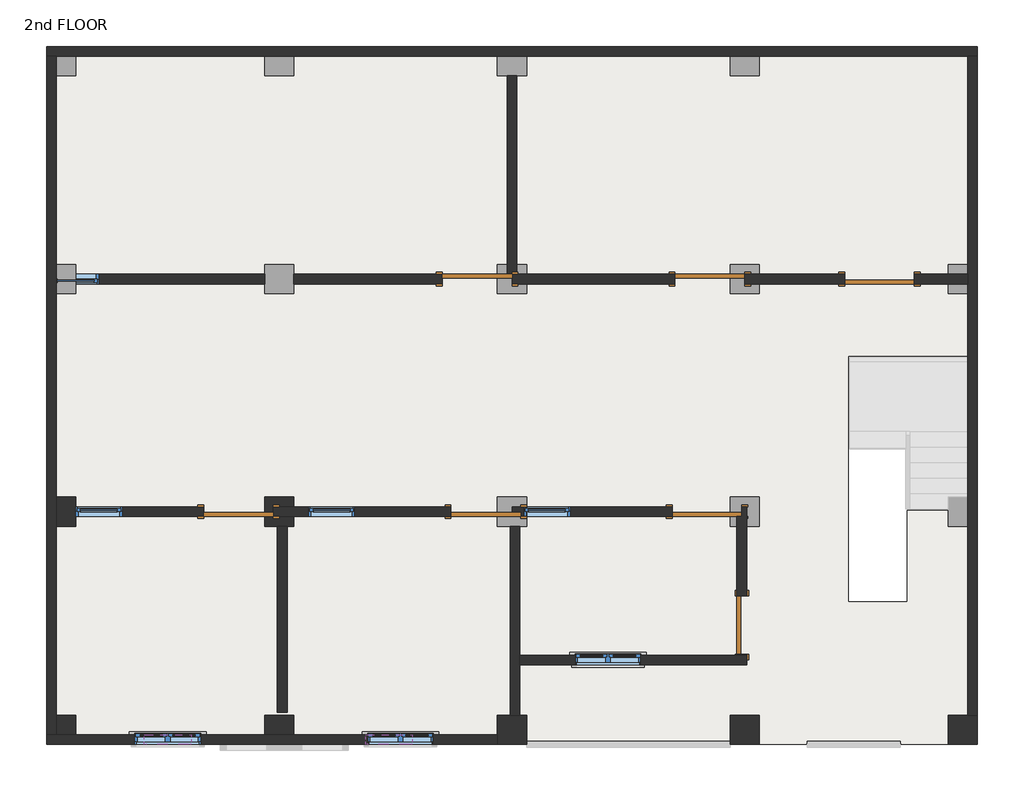
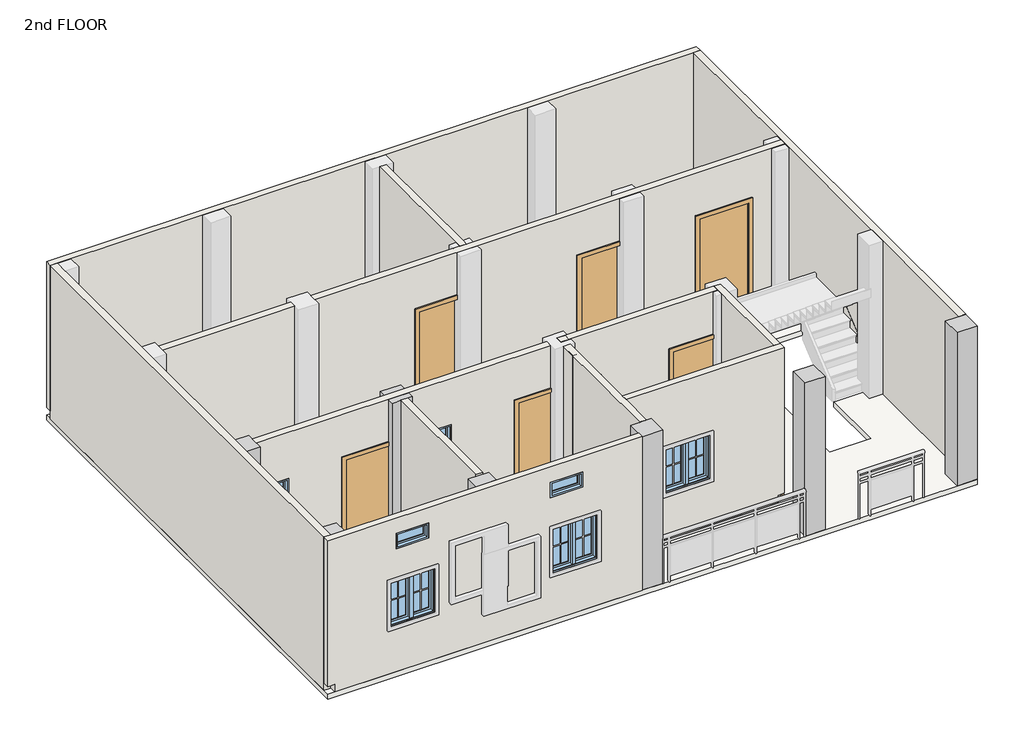
# One storey, part 1 of 2: 15 walls, 9 windows, 7 columns, 7 doors, 1 slab.
"""IFC4 building model written with IfcOpenShell, lengths in millimetres."""

from ifc_helpers import new_model, si_unit, frame, origin, place, context, project, spatial, polyline, outline, extrude, faceted_brep, transform, mapped, element, save
from components import door_e00f436c, door_a1797ceb, window_4c2727af, window_0bf3737e, window_78893e6c, window_0d9958e7

model = new_model("IFC4")

# Units and contexts
model_context = context("Model", 3, world=origin())
ifc_project = project(units=[si_unit("LENGTHUNIT", "METRE", prefix="MILLI")], contexts=[model_context])

# Site, building, storey
site = spatial("IfcSite", under=ifc_project)
building = spatial("IfcBuilding", under=site)
storey = spatial("IfcBuildingStorey", under=building, Name="2nd FLOOR", Elevation=5943.6)

# Columns
placement = place(None, origin())
element("IfcColumn", 1, ObjectType="column family : column family", at=placement, inside=storey, context=model_context, shape_type="Brep", body=[
    faceted_brep([(-12957.097125, 2867.2065522, 5948.6), (-12576.097125, 2867.2065522, 5948.6), (-12576.097125, 2740.2065522, 5948.6), (-12842.797125, 2740.2065522, 5948.6), (-12957.097125, 2740.2065522, 5948.6), (-12576.097125, 2486.2065522, 8986.6), (-12576.097125, 2486.2065522, 5948.6), (-12576.097125, 2613.2065522, 5948.6), (-12576.097125, 2613.2065522, 6096.0), (-12576.097125, 2613.2065522, 8986.6), (-12957.097125, 2486.2065522, 5948.6), (-12957.097125, 2486.2065522, 8986.6), (-12957.097125, 2613.2065522, 8986.6), (-12957.097125, 2613.2065522, 8077.2), (-12957.097125, 2740.2065522, 8077.2), (-12957.097125, 2740.2065522, 8986.6), (-12957.097125, 2867.2065522, 8986.6), (-12957.097125, 2740.2065522, 6096.0), (-12957.097125, 2613.2065522, 6096.0), (-12957.097125, 2613.2065522, 5948.6), (-12576.097125, 2867.2065522, 8986.6), (-12842.797125, 2613.2065522, 5948.6), (-12842.797125, 2613.2065522, 6096.0), (-12842.797125, 2613.2065522, 8077.2), (-12576.097125, 2740.2065522, 6096.0), (-12576.097125, 2740.2065522, 8986.6), (-12842.797125, 2740.2065522, 8077.2), (-12842.797125, 2740.2065522, 6096.0)], [[[0, 1, 2, 3, 4]], [[5, 6, 7, 8, 9]], [[10, 6, 5, 11]], [[10, 11, 12, 13, 14, 15, 16, 0, 4, 17, 18, 19]], [[1, 0, 16, 20]], [[11, 5, 9, 12]], [[7, 21, 22, 23, 13, 12, 9, 8]], [[3, 2, 24, 25, 15, 14, 26, 27]], [[1, 20, 25, 24, 2]], [[20, 16, 15, 25]], [[23, 26, 14, 13]], [[26, 23, 22, 27]], [[18, 22, 21, 19]], [[27, 17, 4, 3]], [[22, 18, 17, 27]], [[6, 10, 19, 21, 7]]]),
])
element("IfcColumn", 2, ObjectType="column family : column family", at=placement, inside=storey, context=model_context, shape_type="SweptSolid", body=[
    extrude(outline(polyline([(-15433.597125, 2867.2065522), (-15433.597125, 2486.2065522), (-15687.597125, 2486.2065522), (-15687.597125, 2867.2065522), (-15433.597125, 2867.2065522)])), frame((0.0, 0.0, 5948.6), z_axis=(0.0, 0.0, 1.0), x_axis=(1.0, 0.0, 0.0)), (0.0, 0.0, 1.0), 3038.0),
])
element("IfcColumn", 3, ObjectType="column family : column family", at=placement, inside=storey, context=model_context, shape_type="Brep", body=[
    faceted_brep([(-15433.597125, 9.7065522, 5948.6), (-15433.597125, 9.7065522, 8986.6), (-15433.597125, -244.2934478, 8986.6), (-15433.597125, -244.2934478, 6096.0), (-15433.597125, -244.2934478, 5948.6), (-15687.597125, 9.7065522, 5948.6), (-15687.597125, 9.7065522, 8986.6), (-15687.597125, -244.2934478, 8986.6), (-15687.597125, -244.2934478, 5948.6), (-15687.597125, -244.2934478, 6096.0)], [[[0, 1, 2, 3, 4]], [[1, 0, 5, 6]], [[2, 1, 6, 7]], [[8, 4, 3, 2, 7, 9]], [[5, 8, 9, 7, 6]], [[0, 4, 8, 5]]]),
])
element("IfcColumn", 4, ObjectType="column family : column family", at=placement, inside=storey, context=model_context, shape_type="Brep", body=[
    faceted_brep([(-3622.597125, 9.7065522, 5948.6), (-3622.597125, -371.2934478, 5948.6), (-4003.597125, -371.2934478, 5948.6), (-4003.597125, 9.7065522, 5948.6), (-3622.597125, 9.7065522, 8986.6), (-3622.597125, -371.2934478, 8986.6), (-3622.597125, 9.7065522, 6096.0), (-4003.597125, -371.2934478, 8986.6), (-4003.597125, 9.7065522, 8986.6)], [[[0, 1, 2, 3]], [[4, 5, 1, 0, 6]], [[5, 7, 2, 1]], [[7, 8, 3, 2]], [[8, 4, 6, 0, 3]], [[4, 8, 7, 5]]]),
])
element("IfcColumn", 5, ObjectType="column family : column family", at=placement, inside=storey, context=model_context, shape_type="SweptSolid", body=[
    extrude(outline(polyline([(-6480.097125, 9.7065522), (-6480.097125, -371.2934478), (-6861.097125, -371.2934478), (-6861.097125, 9.7065522), (-6480.097125, 9.7065522)])), frame((0.0, 0.0, 5948.6), z_axis=(0.0, 0.0, 1.0), x_axis=(1.0, 0.0, 0.0)), (0.0, 0.0, 1.0), 3038.0),
])
element("IfcColumn", 6, ObjectType="column family : column family", at=placement, inside=storey, context=model_context, shape_type="Brep", body=[
    faceted_brep([(-9528.097125, 9.7065522, 5948.6), (-9528.097125, -371.2934478, 5948.6), (-9909.097125, -371.2934478, 5948.6), (-9909.097125, 9.7065522, 5948.6), (-9528.097125, 9.7065522, 8986.6), (-9528.097125, -371.2934478, 8986.6), (-9909.097125, -371.2934478, 8986.6), (-9909.097125, -371.2934478, 6096.0), (-9909.097125, 9.7065522, 8986.6)], [[[0, 1, 2, 3]], [[4, 5, 1, 0]], [[5, 6, 7, 2, 1]], [[6, 8, 3, 2, 7]], [[8, 4, 0, 3]], [[4, 8, 6, 5]]]),
])
element("IfcColumn", 7, ObjectType="column family : column family", at=placement, inside=storey, context=model_context, shape_type="SweptSolid", body=[
    extrude(outline(polyline([(-12957.097125, 9.7065522), (-12576.097125, 9.7065522), (-12576.097125, -244.2934478), (-12957.097125, -244.2934478), (-12957.097125, 9.7065522)])), frame((0.0, 0.0, 5948.6), z_axis=(0.0, 0.0, 1.0), x_axis=(1.0, 0.0, 0.0)), (0.0, 0.0, 1.0), 3038.0),
])

# Doors
door_shape = door_e00f436c(model_context)
element("IfcDoor", 8, ObjectType="Single-Flush : 30\" x 80\"", at=placement, inside=storey, context=model_context, shape_type="MappedRepresentation", body=[
    mapped(door_shape, transform((-6708.697125, 1190.8065522, 5943.6), x_axis=(0.0, -1.0, 0.0), y_axis=(1.0, 0.0, 0.0), z_axis=(0.0, 0.0, 1.0))),
])
door_2_shape = door_a1797ceb(model_context)
element("IfcDoor", 9, ObjectType="Single-Flush : 36\" x 84\"", at=placement, inside=storey, context=model_context, shape_type="MappedRepresentation", body=[
    mapped(door_2_shape, transform((-10175.797125, 5724.7065522, 5943.6), x_axis=(1.0, 0.0, 0.0), y_axis=(0.0, 1.0, 0.0), z_axis=(0.0, 0.0, 1.0))),
])
element("IfcDoor", 10, ObjectType="Single-Flush : 36\" x 84\"", at=placement, inside=storey, context=model_context, shape_type="MappedRepresentation", body=[
    mapped(door_2_shape, transform((-10061.497125, 2676.7065522, 5943.6), x_axis=(-1.0, 0.0, 0.0), y_axis=(0.0, -1.0, 0.0), z_axis=(0.0, 0.0, 1.0))),
])
element("IfcDoor", 11, ObjectType="Single-Flush : 36\" x 84\"", at=placement, inside=storey, context=model_context, shape_type="MappedRepresentation", body=[
    mapped(door_2_shape, transform((-13299.997125, 2676.7065522, 5943.6), x_axis=(-1.0, 0.0, 0.0), y_axis=(0.0, -1.0, 0.0), z_axis=(0.0, 0.0, 1.0))),
])
element("IfcDoor", 12, ObjectType="Single-Flush : 36\" x 84\"", at=placement, inside=storey, context=model_context, shape_type="MappedRepresentation", body=[
    mapped(door_2_shape, transform((-7127.797125, 5724.7065522, 5943.6), x_axis=(1.0, 0.0, 0.0), y_axis=(0.0, 1.0, 0.0), z_axis=(0.0, 0.0, 1.0))),
])
element("IfcDoor", 13, ObjectType="Single-Flush : 36\" x 84\"", at=placement, inside=storey, context=model_context, shape_type="MappedRepresentation", body=[
    mapped(door_2_shape, transform((-7165.897125, 2676.7065522, 5943.6), x_axis=(-1.0, 0.0, 0.0), y_axis=(0.0, -1.0, 0.0), z_axis=(0.0, 0.0, 1.0))),
])
element("IfcDoor", 14, ObjectType="Single-Flush : 36\" x 84\"", at=placement, inside=storey, context=model_context, shape_type="MappedRepresentation", body=[
    mapped(door_2_shape, transform((-4905.297125, 5724.7065522, 5943.6), x_axis=(-1.0, 0.0, 0.0), y_axis=(0.0, -1.0, 0.0), z_axis=(0.0, 0.0, 1.0))),
])

# Slab
element("IfcSlab", 15, ObjectType="Generic - 4\"", at=placement, inside=storey, context=model_context, shape_type="SweptSolid", body=[
    extrude(outline(polyline([(-3622.597125, 8772.7065522), (-3622.597125, -371.2934478), (-15814.597125, -371.2934478), (-15814.597125, 8772.7065522), (-3622.597125, 8772.7065522)]), holes=[polyline([(-3734.357125, 4711.0719226), (-5310.2646464, 4711.0719226), (-5310.2646464, 1502.3126957), (-4547.7736682, 1502.3126957), (-4547.7736682, 2699.911213), (-3734.357125, 2699.911213), (-3734.357125, 4711.0719226)])]), frame((0.0, 0.0, 5842.0), z_axis=(0.0, 0.0, 1.0), x_axis=(1.0, 0.0, 0.0)), (0.0, 0.0, 1.0), 101.6),
])

# Walls
element("IfcWall", 16, ObjectType="Generic - 5\"", at=placement, inside=storey, context=model_context, shape_type="Brep", body=[
    faceted_brep([(-15687.597125, 8645.7065522, 5943.6), (-3749.597125, 8645.7065522, 5943.6), (-3749.597125, 8645.7065522, 6096.0), (-3622.597125, 8645.7065522, 6096.0), (-3622.597125, 8645.7065522, 8991.6), (-3749.597125, 8645.7065522, 8991.6), (-15687.597125, 8645.7065522, 8991.6), (-15814.597125, 8645.7065522, 8991.6), (-15814.597125, 8645.7065522, 6096.0), (-15687.597125, 8645.7065522, 6096.0), (-15687.597125, 8645.7065522, 6091.0), (-15687.597125, 8645.7065522, 5948.6), (-15687.597125, 8772.7065522, 5943.6), (-15687.597125, 8772.7065522, 6096.0), (-15814.597125, 8772.7065522, 6096.0), (-15814.597125, 8772.7065522, 8991.6), (-3622.597125, 8772.7065522, 8991.6), (-3622.597125, 8772.7065522, 6096.0), (-3749.597125, 8772.7065522, 6096.0), (-3749.597125, 8772.7065522, 5943.6)], [[[0, 1, 2, 3, 4, 5, 6, 7, 8, 9, 10, 11]], [[12, 13, 14, 15, 16, 17, 18, 19]], [[1, 0, 12, 19]], [[7, 6, 5, 4, 16, 15]], [[8, 14, 13, 9]], [[0, 11, 10, 9, 13, 12]], [[8, 7, 15, 14]], [[17, 3, 2, 18]], [[2, 1, 19, 18]], [[4, 3, 17, 16]]]),
])
element("IfcWall", 17, ObjectType="Generic - 5\"", at=placement, inside=storey, context=model_context, shape_type="Brep", body=[
    faceted_brep([(-3749.597125, 8645.7065522, 8991.6), (-3749.597125, 8645.7065522, 5943.6), (-3749.597125, 5788.2065522, 5943.6), (-3749.597125, 5661.2065522, 5943.6), (-3749.597125, 9.7065522, 5943.6), (-3749.597125, 9.7065522, 8991.6), (-3749.597125, 5661.2065522, 8991.6), (-3749.597125, 5788.2065522, 8991.6), (-3622.597125, 8645.7065522, 5943.6), (-3622.597125, 8645.7065522, 6096.0), (-3622.597125, 8645.7065522, 8991.6), (-3622.597125, 9.7065522, 8991.6), (-3622.597125, 9.7065522, 8986.6), (-3622.597125, 9.7065522, 6091.0), (-3622.597125, 9.7065522, 5948.6), (-3622.597125, 9.7065522, 5943.6)], [[[0, 1, 2, 3, 4, 5, 6, 7]], [[8, 9, 10, 11, 12, 13, 14, 15]], [[4, 3, 2, 1, 8, 15]], [[5, 4, 15, 14, 13, 12, 11]], [[0, 7, 6, 5, 11, 10]], [[0, 10, 9, 8, 1]]]),
])
element("IfcWall", 18, ObjectType="Generic - 5\"", at=placement, inside=storey, context=model_context, shape_type="Brep", body=[
    faceted_brep([(-9909.097125, -244.2934478, 5943.6), (-15687.597125, -244.2934478, 5943.6), (-15687.597125, -244.2934478, 5948.6), (-15687.597125, -244.2934478, 6091.0), (-15687.597125, -244.2934478, 6096.0), (-15814.597125, -244.2934478, 6096.0), (-15814.597125, -244.2934478, 8991.6), (-15687.597125, -244.2934478, 8991.6), (-9909.097125, -244.2934478, 8991.6), (-13795.297125, -244.2934478, 7772.4), (-14658.897125, -244.2934478, 7772.4), (-14658.897125, -244.2934478, 6858.0), (-13795.297125, -244.2934478, 6858.0), (-10747.297125, -244.2934478, 7772.4), (-11610.897125, -244.2934478, 7772.4), (-11610.897125, -244.2934478, 6858.0), (-10747.297125, -244.2934478, 6858.0), (-13922.297125, -244.2934478, 8686.8), (-14531.897125, -244.2934478, 8686.8), (-14531.897125, -244.2934478, 8382.0), (-13922.297125, -244.2934478, 8382.0), (-11026.697125, -244.2934478, 8686.8), (-11636.297125, -244.2934478, 8686.8), (-11636.297125, -244.2934478, 8382.0), (-11026.697125, -244.2934478, 8382.0), (-9909.097125, -371.2934478, 5943.6), (-9909.097125, -371.2934478, 5948.6), (-9909.097125, -371.2934478, 6091.0), (-9909.097125, -371.2934478, 8986.6), (-9909.097125, -371.2934478, 8991.6), (-15814.597125, -371.2934478, 8991.6), (-15814.597125, -371.2934478, 6096.0), (-15687.597125, -371.2934478, 6096.0), (-15687.597125, -371.2934478, 5943.6), (-13795.297125, -371.2934478, 7772.4), (-13795.297125, -371.2934478, 6858.0), (-14658.897125, -371.2934478, 6858.0), (-14658.897125, -371.2934478, 7772.4), (-10747.297125, -371.2934478, 7772.4), (-10747.297125, -371.2934478, 6858.0), (-11610.897125, -371.2934478, 6858.0), (-11610.897125, -371.2934478, 7772.4), (-13922.297125, -371.2934478, 8686.8), (-13922.297125, -371.2934478, 8382.0), (-14531.897125, -371.2934478, 8382.0), (-14531.897125, -371.2934478, 8686.8), (-11026.697125, -371.2934478, 8686.8), (-11026.697125, -371.2934478, 8382.0), (-11636.297125, -371.2934478, 8382.0), (-11636.297125, -371.2934478, 8686.8)], [[[0, 1, 2, 3, 4, 5, 6, 7, 8], [9, 10, 11, 12], [13, 14, 15, 16], [17, 18, 19, 20], [21, 22, 23, 24]], [[25, 26, 27, 28, 29, 30, 31, 32, 33], [34, 35, 36, 37], [38, 39, 40, 41], [42, 43, 44, 45], [46, 47, 48, 49]], [[1, 0, 25, 33]], [[8, 7, 6, 30, 29]], [[0, 8, 29, 28, 27, 26, 25]], [[35, 34, 9, 12]], [[36, 35, 12, 11]], [[37, 36, 11, 10]], [[34, 37, 10, 9]], [[39, 38, 13, 16]], [[40, 39, 16, 15]], [[41, 40, 15, 14]], [[38, 41, 14, 13]], [[43, 42, 17, 20]], [[44, 43, 20, 19]], [[45, 44, 19, 18]], [[42, 45, 18, 17]], [[47, 46, 21, 24]], [[48, 47, 24, 23]], [[49, 48, 23, 22]], [[46, 49, 22, 21]], [[31, 5, 4, 32]], [[4, 3, 2, 1, 33, 32]], [[6, 5, 31, 30]]]),
])
element("IfcWall", 19, ObjectType="Generic - 5\"", at=placement, inside=storey, context=model_context, shape_type="Brep", body=[
    faceted_brep([(-15687.597125, -244.2934478, 8991.6), (-15687.597125, -244.2934478, 8986.6), (-15687.597125, -244.2934478, 6091.0), (-15687.597125, -244.2934478, 5948.6), (-15687.597125, -244.2934478, 5943.6), (-15687.597125, 8645.7065522, 5943.6), (-15687.597125, 8645.7065522, 5948.6), (-15687.597125, 8645.7065522, 6091.0), (-15687.597125, 8645.7065522, 8986.6), (-15687.597125, 8645.7065522, 8991.6), (-15814.597125, -244.2934478, 5943.6), (-15814.597125, -244.2934478, 6096.0), (-15814.597125, -244.2934478, 8991.6), (-15814.597125, 8645.7065522, 8991.6), (-15814.597125, 8645.7065522, 6096.0), (-15814.597125, 8645.7065522, 5943.6)], [[[0, 1, 2, 3, 4, 5, 6, 7, 8, 9]], [[10, 11, 12, 13, 14, 15]], [[5, 4, 10, 15]], [[0, 9, 13, 12]], [[5, 15, 14, 13, 9, 8, 7, 6]], [[0, 12, 11, 10, 4, 3, 2, 1]]]),
])
element("IfcWall", 20, ObjectType="Generic - 5\"", at=placement, inside=storey, context=model_context, shape_type="SweptSolid", body=[
    extrude(outline(polyline([(5943.6, -15433.597125), (5943.6, -12957.097125), (8991.6, -12957.097125), (8991.6, -15433.597125), (8077.2, -15433.597125), (8077.2, -15128.797125), (6248.4, -15128.797125), (6248.4, -15433.597125), (5943.6, -15433.597125)])), frame((0.0, 5661.2065522, 0.0), z_axis=(0.0, 1.0, 0.0), x_axis=(0.0, 0.0, 1.0)), (0.0, 0.0, 1.0), 127.0),
])
element("IfcWall", 21, ObjectType="Generic - 5\"", at=placement, inside=storey, context=model_context, shape_type="Brep", body=[
    faceted_brep([(-9782.097125, 8391.7065522, 5943.6), (-9782.097125, 5788.2065522, 5943.6), (-9782.097125, 5788.2065522, 5948.6), (-9782.097125, 5788.2065522, 6091.0), (-9782.097125, 5788.2065522, 6096.0), (-9782.097125, 5788.2065522, 8077.2), (-9782.097125, 5788.2065522, 8986.6), (-9782.097125, 5788.2065522, 8991.6), (-9782.097125, 8391.7065522, 8991.6), (-9655.097125, 8391.7065522, 5943.6), (-9655.097125, 8391.7065522, 8991.6), (-9655.097125, 5788.2065522, 8991.6), (-9655.097125, 5788.2065522, 8986.6), (-9655.097125, 5788.2065522, 6091.0), (-9655.097125, 5788.2065522, 5948.6), (-9655.097125, 5788.2065522, 5943.6), (-9718.597125, 5788.2065522, 5943.6)], [[[0, 1, 2, 3, 4, 5, 6, 7, 8]], [[9, 10, 11, 12, 13, 14, 15]], [[1, 0, 9, 15, 16]], [[8, 7, 11, 10]], [[0, 8, 10, 9]], [[1, 16, 15, 14, 13, 12, 11, 7, 6, 5, 4, 3, 2]]]),
])
element("IfcWall", 22, ObjectType="Generic - 5\"", at=placement, inside=storey, context=model_context, shape_type="Brep", body=[
    faceted_brep([(-6670.597125, 5661.2065522, 5943.6), (-5362.497125, 5661.2065522, 5943.6), (-5362.497125, 5661.2065522, 8077.2), (-4448.097125, 5661.2065522, 8077.2), (-4448.097125, 5661.2065522, 5943.6), (-3749.597125, 5661.2065522, 5943.6), (-3749.597125, 5661.2065522, 5948.6), (-3749.597125, 5661.2065522, 6091.0), (-3749.597125, 5661.2065522, 8986.6), (-3749.597125, 5661.2065522, 8991.6), (-12576.097125, 5661.2065522, 8991.6), (-12576.097125, 5661.2065522, 5943.6), (-10632.997125, 5661.2065522, 5943.6), (-10632.997125, 5661.2065522, 8077.2), (-9909.097125, 5661.2065522, 8077.2), (-9718.597125, 5661.2065522, 8077.2), (-9718.597125, 5661.2065522, 6096.0), (-9718.597125, 5661.2065522, 5943.6), (-7584.997125, 5661.2065522, 5943.6), (-7584.997125, 5661.2065522, 8077.2), (-6861.097125, 5661.2065522, 8077.2), (-6670.597125, 5661.2065522, 8077.2), (-6670.597125, 5661.2065522, 6096.0), (-5362.497125, 5788.2065522, 8077.2), (-5362.497125, 5788.2065522, 5943.6), (-6670.597125, 5788.2065522, 5943.6), (-6670.597125, 5788.2065522, 6096.0), (-6670.597125, 5788.2065522, 8077.2), (-6861.097125, 5788.2065522, 8077.2), (-7584.997125, 5788.2065522, 8077.2), (-7584.997125, 5788.2065522, 5943.6), (-9655.097125, 5788.2065522, 5943.6), (-9718.597125, 5788.2065522, 5943.6), (-9718.597125, 5788.2065522, 6096.0), (-9718.597125, 5788.2065522, 8077.2), (-9782.097125, 5788.2065522, 8077.2), (-9909.097125, 5788.2065522, 8077.2), (-10632.997125, 5788.2065522, 8077.2), (-10632.997125, 5788.2065522, 5943.6), (-12576.097125, 5788.2065522, 5943.6), (-12576.097125, 5788.2065522, 8991.6), (-9782.097125, 5788.2065522, 8991.6), (-9655.097125, 5788.2065522, 8991.6), (-3749.597125, 5788.2065522, 8991.6), (-3749.597125, 5788.2065522, 8986.6), (-3749.597125, 5788.2065522, 6091.0), (-3749.597125, 5788.2065522, 5948.6), (-3749.597125, 5788.2065522, 5943.6), (-4448.097125, 5788.2065522, 5943.6), (-4448.097125, 5788.2065522, 8077.2)], [[[0, 1, 2, 3, 4, 5, 6, 7, 8, 9, 10, 11, 12, 13, 14, 15, 16, 17, 18, 19, 20, 21, 22]], [[23, 24, 25, 26, 27, 28, 29, 30, 31, 32, 33, 34, 35, 36, 37, 38, 39, 40, 41, 42, 43, 44, 45, 46, 47, 48, 49]], [[12, 11, 39, 38]], [[18, 17, 32, 31, 30]], [[48, 47, 5, 4]], [[25, 24, 1, 0]], [[10, 9, 43, 42, 41, 40]], [[11, 10, 40, 39]], [[34, 33, 32, 17, 16, 15]], [[37, 36, 35, 34, 15, 14, 13]], [[38, 37, 13, 12]], [[27, 26, 25, 0, 22, 21]], [[29, 28, 27, 21, 20, 19]], [[30, 29, 19, 18]], [[2, 1, 24, 23]], [[3, 2, 23, 49]], [[4, 3, 49, 48]], [[5, 47, 46, 45, 44, 43, 9, 8, 7, 6]]]),
])
element("IfcWall", 23, ObjectType="Generic - 5\"", at=placement, inside=storey, context=model_context, shape_type="Brep", body=[
    faceted_brep([(-14823.997125, 2613.2065522, 6248.4), (-15433.597125, 2613.2065522, 6248.4), (-15433.597125, 2613.2065522, 5943.6), (-13757.197125, 2613.2065522, 5943.6), (-13757.197125, 2613.2065522, 8077.2), (-12957.097125, 2613.2065522, 8077.2), (-12842.797125, 2613.2065522, 8077.2), (-12842.797125, 2613.2065522, 6096.0), (-12842.797125, 2613.2065522, 5943.6), (-10518.697125, 2613.2065522, 5943.6), (-10518.697125, 2613.2065522, 8077.2), (-9909.097125, 2613.2065522, 8077.2), (-9909.097125, 2613.2065522, 8991.6), (-15433.597125, 2613.2065522, 8991.6), (-15433.597125, 2613.2065522, 8077.2), (-14823.997125, 2613.2065522, 8077.2), (-12385.597125, 2613.2065522, 8077.2), (-11775.997125, 2613.2065522, 8077.2), (-11775.997125, 2613.2065522, 6248.4), (-12385.597125, 2613.2065522, 6248.4), (-15433.597125, 2740.2065522, 5943.6), (-15433.597125, 2740.2065522, 6248.4), (-14823.997125, 2740.2065522, 6248.4), (-14823.997125, 2740.2065522, 8077.2), (-15433.597125, 2740.2065522, 8077.2), (-15433.597125, 2740.2065522, 8991.6), (-9909.097125, 2740.2065522, 8991.6), (-9909.097125, 2740.2065522, 8077.2), (-10518.697125, 2740.2065522, 8077.2), (-10518.697125, 2740.2065522, 5943.6), (-12842.797125, 2740.2065522, 5943.6), (-12842.797125, 2740.2065522, 6096.0), (-12842.797125, 2740.2065522, 8077.2), (-12957.097125, 2740.2065522, 8077.2), (-13757.197125, 2740.2065522, 8077.2), (-13757.197125, 2740.2065522, 5943.6), (-12385.597125, 2740.2065522, 8077.2), (-12385.597125, 2740.2065522, 6248.4), (-11775.997125, 2740.2065522, 6248.4), (-11775.997125, 2740.2065522, 8077.2)], [[[0, 1, 2, 3, 4, 5, 6, 7, 8, 9, 10, 11, 12, 13, 14, 15], [16, 17, 18, 19]], [[20, 21, 22, 23, 24, 25, 26, 27, 28, 29, 30, 31, 32, 33, 34, 35], [36, 37, 38, 39]], [[30, 29, 9, 8]], [[20, 35, 3, 2]], [[26, 12, 11, 27]], [[13, 12, 26, 25]], [[14, 13, 25, 24]], [[2, 1, 21, 20]], [[28, 10, 9, 29]], [[10, 28, 27, 11]], [[4, 3, 35, 34]], [[6, 5, 4, 34, 33, 32]], [[8, 7, 6, 32, 31, 30]], [[22, 21, 1, 0]], [[23, 22, 0, 15]], [[24, 23, 15, 14]], [[37, 36, 16, 19]], [[38, 37, 19, 18]], [[39, 38, 18, 17]], [[36, 39, 17, 16]]]),
])
element("IfcWall", 24, ObjectType="Generic - 5\"", at=placement, inside=storey, context=model_context, shape_type="Brep", body=[
    faceted_brep([(-9616.997125, 9.7065522, 5943.6), (-9616.997125, 670.1065522, 5943.6), (-9616.997125, 797.1065522, 5943.6), (-9616.997125, 2486.2065522, 5943.6), (-9616.997125, 2486.2065522, 8991.6), (-9616.997125, 797.1065522, 8991.6), (-9616.997125, 670.1065522, 8991.6), (-9616.997125, 9.7065522, 8991.6), (-9743.997125, 9.7065522, 5943.6), (-9743.997125, 9.7065522, 8991.6), (-9743.997125, 2486.2065522, 8991.6), (-9743.997125, 2486.2065522, 5943.6)], [[[0, 1, 2, 3, 4, 5, 6, 7]], [[8, 9, 10, 11]], [[3, 2, 1, 0, 8, 11]], [[4, 3, 11, 10]], [[7, 6, 5, 4, 10, 9]], [[0, 7, 9, 8]]]),
])
element("IfcWall", 25, ObjectType="Generic - 5\"", at=placement, inside=storey, context=model_context, shape_type="SweptSolid", body=[
    extrude(outline(polyline([(-9743.997125, 2181.4065522), (-9743.997125, 2486.2065522), (-9616.997125, 2486.2065522), (-9616.997125, 2181.4065522), (-9743.997125, 2181.4065522)])), frame((0.0, 0.0, 5943.6), z_axis=(0.0, 0.0, 1.0), x_axis=(1.0, 0.0, 0.0)), (0.0, 0.0, 1.0), 3048.0),
])
element("IfcWall", 26, ObjectType="Generic - 5\"", at=placement, inside=storey, context=model_context, shape_type="Brep", body=[
    faceted_brep([(-6772.197125, 2613.2065522, 8991.6), (-9718.597125, 2613.2065522, 8991.6), (-9718.597125, 2613.2065522, 8986.6), (-9718.597125, 2613.2065522, 6091.0), (-9718.597125, 2613.2065522, 5948.6), (-9718.597125, 2613.2065522, 5943.6), (-7623.097125, 2613.2065522, 5943.6), (-7623.097125, 2613.2065522, 8077.2), (-6861.097125, 2613.2065522, 8077.2), (-6772.197125, 2613.2065522, 8077.2), (-6772.197125, 2613.2065522, 8986.6), (-9566.197125, 2613.2065522, 8077.2), (-9528.097125, 2613.2065522, 8077.2), (-8956.597125, 2613.2065522, 8077.2), (-8956.597125, 2613.2065522, 6248.4), (-9528.097125, 2613.2065522, 6248.4), (-9566.197125, 2613.2065522, 6248.4), (-9718.597125, 2740.2065522, 8991.6), (-6772.197125, 2740.2065522, 8991.6), (-6772.197125, 2740.2065522, 8077.2), (-6861.097125, 2740.2065522, 8077.2), (-7623.097125, 2740.2065522, 8077.2), (-7623.097125, 2740.2065522, 5943.6), (-9718.597125, 2740.2065522, 5943.6), (-9718.597125, 2740.2065522, 5948.6), (-9718.597125, 2740.2065522, 6091.0), (-9718.597125, 2740.2065522, 8986.6), (-9566.197125, 2740.2065522, 8077.2), (-9566.197125, 2740.2065522, 6248.4), (-9528.097125, 2740.2065522, 6248.4), (-8956.597125, 2740.2065522, 6248.4), (-8956.597125, 2740.2065522, 8077.2), (-9528.097125, 2740.2065522, 8077.2)], [[[0, 1, 2, 3, 4, 5, 6, 7, 8, 9, 10], [11, 12, 13, 14, 15, 16]], [[17, 18, 19, 20, 21, 22, 23, 24, 25, 26], [27, 28, 29, 30, 31, 32]], [[5, 23, 22, 6]], [[1, 0, 18, 17]], [[5, 4, 3, 2, 1, 17, 26, 25, 24, 23]], [[28, 27, 11, 16]], [[30, 29, 28, 16, 15, 14]], [[31, 30, 14, 13]], [[27, 32, 31, 13, 12, 11]], [[21, 7, 6, 22]], [[7, 21, 20, 19, 9, 8]], [[18, 0, 10, 9, 19]]]),
])
element("IfcWall", 27, ObjectType="Generic - 5\"", at=placement, inside=storey, context=model_context, shape_type="Brep", body=[
    faceted_brep([(-6645.197125, 797.1065522, 5943.6), (-6645.197125, 809.8065522, 5943.6), (-6645.197125, 809.8065522, 7975.6), (-6645.197125, 1571.8065522, 7975.6), (-6645.197125, 1571.8065522, 5943.6), (-6645.197125, 2613.2065522, 5943.6), (-6645.197125, 2613.2065522, 6096.0), (-6645.197125, 2740.2065522, 6096.0), (-6645.197125, 2740.2065522, 8986.6), (-6645.197125, 2740.2065522, 8991.6), (-6645.197125, 797.1065522, 8991.6), (-6645.197125, 797.1065522, 6096.0), (-6772.197125, 809.8065522, 7975.6), (-6772.197125, 809.8065522, 5943.6), (-6772.197125, 797.1065522, 5943.6), (-6772.197125, 797.1065522, 8991.6), (-6772.197125, 2613.2065522, 8991.6), (-6772.197125, 2740.2065522, 8991.6), (-6772.197125, 2740.2065522, 8077.2), (-6772.197125, 2613.2065522, 8077.2), (-6772.197125, 2613.2065522, 6091.0), (-6772.197125, 2613.2065522, 5948.6), (-6772.197125, 2613.2065522, 5943.6), (-6772.197125, 1571.8065522, 5943.6), (-6772.197125, 1571.8065522, 7975.6), (-6708.697125, 2613.2065522, 5943.6), (-6708.697125, 2740.2065522, 8077.2), (-6708.697125, 2613.2065522, 8077.2), (-6708.697125, 2740.2065522, 6096.0), (-6708.697125, 2613.2065522, 6096.0)], [[[0, 1, 2, 3, 4, 5, 6, 7, 8, 9, 10, 11]], [[12, 13, 14, 15, 16, 17, 18, 19, 20, 21, 22, 23, 24]], [[23, 22, 25, 5, 4]], [[14, 13, 1, 0]], [[10, 9, 17, 16, 15]], [[26, 27, 19, 18]], [[27, 26, 28, 29]], [[2, 1, 13, 12]], [[3, 2, 12, 24]], [[4, 3, 24, 23]], [[7, 6, 29, 28]], [[6, 5, 25, 22, 21, 20, 19, 27, 29]], [[9, 8, 7, 28, 26, 18, 17]], [[14, 0, 11, 10, 15]]]),
])
element("IfcWall", 28, ObjectType="Generic - 5\"", at=placement, inside=storey, context=model_context, shape_type="Brep", body=[
    faceted_brep([(-9718.597125, 2613.2065522, 5943.6), (-9566.197125, 2613.2065522, 5943.6), (-9566.197125, 2613.2065522, 6248.4), (-9566.197125, 2613.2065522, 8077.2), (-9566.197125, 2613.2065522, 8991.6), (-9718.597125, 2613.2065522, 8991.6), (-9718.597125, 2613.2065522, 8986.6), (-9718.597125, 2613.2065522, 6091.0), (-9718.597125, 2613.2065522, 5948.6), (-9718.597125, 2740.2065522, 5943.6), (-9718.597125, 2740.2065522, 5948.6), (-9718.597125, 2740.2065522, 6091.0), (-9718.597125, 2740.2065522, 8986.6), (-9718.597125, 2740.2065522, 8991.6), (-9566.197125, 2740.2065522, 8991.6), (-9566.197125, 2740.2065522, 8077.2), (-9566.197125, 2740.2065522, 6248.4), (-9566.197125, 2740.2065522, 5943.6)], [[[0, 1, 2, 3, 4, 5, 6, 7, 8]], [[9, 10, 11, 12, 13, 14, 15, 16, 17]], [[1, 0, 9, 17]], [[4, 3, 2, 1, 17, 16, 15, 14]], [[5, 4, 14, 13]], [[0, 8, 7, 6, 5, 13, 12, 11, 10, 9]]]),
])
element("IfcWall", 29, ObjectType="Generic - 5\"", at=placement, inside=storey, context=model_context, shape_type="SweptSolid", body=[
    extrude(outline(polyline([(-12791.997125, 47.8065522), (-12791.997125, 2486.2065522), (-12664.997125, 2486.2065522), (-12664.997125, 47.8065522), (-12791.997125, 47.8065522)])), frame((0.0, 0.0, 5943.6), z_axis=(0.0, 0.0, 1.0), x_axis=(1.0, 0.0, 0.0)), (0.0, 0.0, 1.0), 3048.0),
])
element("IfcWall", 30, ObjectType="Generic - 5\"", at=placement, inside=storey, context=model_context, shape_type="Brep", body=[
    faceted_brep([(-9616.997125, 670.1065522, 8991.6), (-9616.997125, 670.1065522, 5943.6), (-6772.197125, 670.1065522, 5943.6), (-6772.197125, 670.1065522, 6096.0), (-6645.197125, 670.1065522, 6096.0), (-6645.197125, 670.1065522, 8991.6), (-8029.497125, 670.1065522, 7772.4), (-8029.497125, 670.1065522, 6858.0), (-8893.097125, 670.1065522, 6858.0), (-8893.097125, 670.1065522, 7772.4), (-9616.997125, 797.1065522, 5943.6), (-9616.997125, 797.1065522, 8991.6), (-6772.197125, 797.1065522, 8991.6), (-6645.197125, 797.1065522, 8991.6), (-6645.197125, 797.1065522, 6096.0), (-6772.197125, 797.1065522, 6096.0), (-6772.197125, 797.1065522, 5943.6), (-8029.497125, 797.1065522, 7772.4), (-8893.097125, 797.1065522, 7772.4), (-8893.097125, 797.1065522, 6858.0), (-8029.497125, 797.1065522, 6858.0)], [[[0, 1, 2, 3, 4, 5], [6, 7, 8, 9]], [[10, 11, 12, 13, 14, 15, 16], [17, 18, 19, 20]], [[2, 1, 10, 16]], [[0, 5, 13, 12, 11]], [[7, 6, 17, 20]], [[8, 7, 20, 19]], [[9, 8, 19, 18]], [[6, 9, 18, 17]], [[0, 11, 10, 1]], [[14, 4, 3, 15]], [[3, 2, 16, 15]], [[5, 4, 14, 13]]]),
])

# Windows
window_shape = window_4c2727af(model_context)
element("IfcWindow", 31, ObjectType="Fixed : 24\" x 12\"", at=placement, inside=storey, context=model_context, shape_type="MappedRepresentation", body=[
    mapped(window_shape, transform((-14188.997125, -307.7934478, 7467.6), x_axis=(1.0, 0.0, 0.0), y_axis=(0.0, 1.0, 0.0), z_axis=(0.0, 0.0, 1.0))),
])
element("IfcWindow", 32, ObjectType="Fixed : 24\" x 12\"", at=placement, inside=storey, context=model_context, shape_type="MappedRepresentation", body=[
    mapped(window_shape, transform((-11293.397125, -307.7934478, 7467.6), x_axis=(1.0, 0.0, 0.0), y_axis=(0.0, 1.0, 0.0), z_axis=(0.0, 0.0, 1.0))),
])
window_2_shape = window_0bf3737e(model_context)
element("IfcWindow", 33, ObjectType="Fixed : 24\" x 72\"", at=placement, inside=storey, context=model_context, shape_type="MappedRepresentation", body=[
    mapped(window_2_shape, transform((-15471.697125, 5724.7065522, 5943.6), x_axis=(-1.0, 0.0, 0.0), y_axis=(0.0, -1.0, 0.0), z_axis=(0.0, 0.0, 1.0))),
])
window_3_shape = window_78893e6c(model_context)
element("IfcWindow", 34, ObjectType="Fixed : 24\" x 72\"", at=placement, inside=storey, context=model_context, shape_type="MappedRepresentation", body=[
    mapped(window_3_shape, transform((-15166.897125, 2676.7065522, 5943.6), x_axis=(-1.0, 0.0, 0.0), y_axis=(0.0, -1.0, 0.0), z_axis=(0.0, 0.0, 1.0))),
])
element("IfcWindow", 35, ObjectType="Fixed : 24\" x 72\"", at=placement, inside=storey, context=model_context, shape_type="MappedRepresentation", body=[
    mapped(window_3_shape, transform((-12118.897125, 2676.7065522, 5943.6), x_axis=(-1.0, 0.0, 0.0), y_axis=(0.0, -1.0, 0.0), z_axis=(0.0, 0.0, 1.0))),
])
element("IfcWindow", 36, ObjectType="Fixed : 24\" x 72\"", at=placement, inside=storey, context=model_context, shape_type="MappedRepresentation", body=[
    mapped(window_3_shape, transform((-9299.497125, 2676.7065522, 5943.6), x_axis=(-1.0, 0.0, 0.0), y_axis=(0.0, -1.0, 0.0), z_axis=(0.0, 0.0, 1.0))),
])
window_4_shape = window_0d9958e7(model_context)
element("IfcWindow", 37, ObjectType="Window-Casement-Double : 34\" x 36\"", at=placement, inside=storey, context=model_context, shape_type="MappedRepresentation", body=[
    mapped(window_4_shape, transform((-14227.097125, -307.7934478, 5943.6), x_axis=(1.0, 0.0, 0.0), y_axis=(0.0, 1.0, 0.0), z_axis=(0.0, 0.0, 1.0))),
])
element("IfcWindow", 38, ObjectType="Window-Casement-Double : 34\" x 36\"", at=placement, inside=storey, context=model_context, shape_type="MappedRepresentation", body=[
    mapped(window_4_shape, transform((-11179.097125, -307.7934478, 5943.6), x_axis=(1.0, 0.0, 0.0), y_axis=(0.0, 1.0, 0.0), z_axis=(0.0, 0.0, 1.0))),
])
element("IfcWindow", 39, ObjectType="Window-Casement-Double : 34\" x 36\"", at=placement, inside=storey, context=model_context, shape_type="MappedRepresentation", body=[
    mapped(window_4_shape, transform((-8461.297125, 733.6065522, 5943.6), x_axis=(1.0, 0.0, 0.0), y_axis=(0.0, 1.0, 0.0), z_axis=(0.0, 0.0, 1.0))),
])

save(model, "model.ifc")

# Revit data of these elements
# Type "column family : column family"
#   w2 [instance default] = 0' - 9.88189"
#   w1 [instance default] = 0' - 9.01575"
#   Depth = 1' - 11.62205"
#   Width = 1' - 11.62205"
# Type "Single-Flush : 30\" x 80\""
#   Type Mark = "5"
#   Construction Type Id = "MDOOR"
#   Assembly Code = "C1020"
#   Analytic Construction = "Metal"
#   Thickness = 0' - 2"
#   Heat Transfer Coefficient (U) = 0.651978 BTU/(h·ft²·°F)
#   Height = 6' - 8"
#   Trim Projection Ext = 0' - 1"
#   Trim Projection Int = 0' - 1"
#   Trim Width = 0' - 3"
#   Width = 2' - 6"
#   Define Thermal Properties by = 1
#   Define Thermal Properties by = 1
#   Door Material = Door - Panel
#   Frame Material = Door - Frame
#   Visual Light Transmittance = 0
#   Solar Heat Gain Coefficient = 0
#   Function = (empty or 0)
#   Wall Closure = (empty or 0)
# Type "Single-Flush : 36\" x 84\""
#   Type Mark = "1"
#   Construction Type Id = "MDOOR"
#   Assembly Code = "C1020"
#   Analytic Construction = "Metal"
#   Thickness = 0' - 2"
#   Heat Transfer Coefficient (U) = 0.651978 BTU/(h·ft²·°F)
#   Height = 7' - 0"
#   Trim Projection Ext = 0' - 1"
#   Trim Projection Int = 0' - 1"
#   Trim Width = 0' - 3"
#   Width = 3' - 0"
#   Define Thermal Properties by = 1
#   Define Thermal Properties by = 1
#   Door Material = Door - Panel
#   Frame Material = Door - Frame
#   Visual Light Transmittance = 0
#   Solar Heat Gain Coefficient = 0
#   Function = (empty or 0)
#   Wall Closure = (empty or 0)
# Type "Generic - 4\""
#   Assembly Code = "B1010"
#   Function = 0
#   Layers, outside or top first: 0' - 4" no material (function 1)
# Type "Generic - 5\""
#   Assembly Code = "B2010"
#   Layers, outside or top first: 0' - 5" no material (function 1)
# Type "Fixed : 24\" x 12\""
#   Type Mark = "4"
#   Construction Type Id = "GSP4R"
#   Assembly Code = "B2020100"
#   Analytic Construction = "1/8 in Pilkington single glazing"
#   Visual Light Transmittance = 0.9
#   Solar Heat Gain Coefficient = 0.78
#   Heat Transfer Coefficient (U) = 0.6496 BTU/(h·ft²·°F)
#   Height = 1' - 0"
#   Default Sill Height = 3' - 0"
#   Width = 2' - 0"
#   Window Inset = 0' - 0 3/4"
#   Define Thermal Properties by = 1
#   Define Thermal Properties by = 1
#   Glass Pane Material = Glass
#   Sash Material = Sash
#   Wall Closure = (empty or 0)
# Type "Fixed : 24\" x 72\""
#   Type Mark = "7"
#   Construction Type Id = "GSP4R"
#   Assembly Code = "B2020100"
#   Analytic Construction = "1/8 in Pilkington single glazing"
#   Visual Light Transmittance = 0.9
#   Solar Heat Gain Coefficient = 0.78
#   Heat Transfer Coefficient (U) = 0.6496 BTU/(h·ft²·°F)
#   Height = 6' - 0"
#   Default Sill Height = 1' - 0"
#   Width = 2' - 0"
#   Window Inset = 0' - 0 3/4"
#   Define Thermal Properties by = 1
#   Define Thermal Properties by = 1
#   Glass Pane Material = Glass
#   Sash Material = Sash
#   Wall Closure = (empty or 0)
# Type "Window-Casement-Double : 34\" x 36\""
#   Type Mark = "14"
#   Fire Rating = "0.5h"
#   Assembly Code = "B2020100"
#   Analytic Construction = "Double glazing - domestic"
#   Frame Extension [instance default] = 0' - 0 1/4"
#   Window Inset [instance default] = 0' - 0"
#   Wall Thickness [instance default] = 0' - 6"
#   Interior Wall Closure [instance default] = 0' - 2 1/4"
#   Half Width = 1' - 5"
#   Visual Light Transmittance = 0.81
#   Thermal Resistance (R) = 1.8146 (h·ft²·°F)/BTU
#   Solar Heat Gain Coefficient = 0.76
#   Rough Width = 2' - 10 1/2"
#   Rough Height = 3' - 0 1/2"
#   Height = 3' - 0"
#   Heat Transfer Coefficient (U) = 0.5511 BTU/(h·ft²·°F)
#   Exterior Wall Closure [instance default] = 0' - 1 1/4"
#   Extension Jamb [instance default] = 0' - 2 1/4"
#   Default Sill Height = 3' - 0"
#   Width = 2' - 10"
#   Define Thermal Properties by = 0
#   Muntin Visibility = yes
#   Interior Trim Visibility [instance default] = yes
#   Exterior Trim Visibility [instance default] = yes
#   Extension Jamb Visibility [instance default] = yes
#   Interior Trim Material = Wood - Stained
#   Muntin Pattern = Muntin Pattern_2x2 : Muntin Pattern_2x2
#   Interior Trim = Trim-Window-Interior-Flat : Picture Frame
#   Interior Frame Material = Wood - Stained
#   Glass Panel Material = Glass
#   Exterior Trim Material = Clad - White
#   Exterior Trim = Trim-Window-Exterior-Flat : with Sill
#   Exterior Frame Material = Clad - White
#   Wall Closure = (empty or 0)
# Element 1 (IfcColumn, "column family : column family")
#   w2 = 1' - 3"
#   w1 = 1' - 3"
#   Phase Created = New Construction
#   Materials on its faces: "Default Wall", "inside wall"
# Element 2 (IfcColumn, "column family : column family")
#   w2 = 1' - 3"
#   w1 = 0' - 10"
#   Phase Created = New Construction
#   Materials on its faces: "inside wall", "Default Wall"
# Elements 3, 7 (IfcColumn, "column family : column family")
#   w2 = 1' - 3"
#   w1 = 1' - 3"
#   Phase Created = New Construction
#   Materials on its faces: "Default Wall"
# Element 4 (IfcColumn, "column family : column family")
#   w2 = 1' - 3"
#   w1 = 1' - 3"
#   Phase Created = New Construction
#   Materials on its faces: "Clad - White", "Default Wall"
# Element 5 (IfcColumn, "column family : column family")
#   w2 = 1' - 3"
#   w1 = 1' - 3"
#   Phase Created = New Construction
#   Materials on its faces: "out side wall"
# Element 6 (IfcColumn, "column family : column family")
#   w2 = 1' - 3"
#   w1 = 1' - 3"
#   Phase Created = New Construction
#   Materials on its faces: "out side wall", "Default Wall"
# Element 8 (IfcDoor, "Single-Flush : 30\" x 80\"")
#   Phase Created = New Construction
#   Materials on its faces: "Door - Frame", "Door - Panel"
# Elements 9, 10, 11, 12, 13, 14 (IfcDoor, "Single-Flush : 36\" x 84\"")
#   Phase Created = New Construction
#   Materials on its faces: "Door - Frame", "Door - Panel"
# Element 15 (IfcSlab, "Generic - 4\"")
#   Height Offset From Level = 0' - 0"
#   Phase Created = New Construction
#   Materials on its faces: "Default Floor", "Clad - White"
# Element 16 (IfcWall, "Generic - 5\"")
#   Top Offset = 0' - 0"
#   Base Offset = 0' - 0"
#   wall height = 10' - 0"
#   Phase Created = New Construction
#   Base Constraint = 2nd FLOOR
#   Top Constraint = 3rd FLOOR
#   Materials on its faces: "Default Wall", "Clad - White"
# Element 17 (IfcWall, "Generic - 5\"")
#   Top Offset = 0' - 0"
#   Base Offset = 0' - 0"
#   wall height = 10' - 0"
#   Phase Created = New Construction
#   Base Constraint = 2nd FLOOR
#   Top Constraint = 3rd FLOOR
#   Materials on its faces: "Default Wall", "grey", "Clad - White"
# Element 18 (IfcWall, "Generic - 5\"")
#   Top Offset = 0' - 0"
#   Base Offset = 0' - 0"
#   wall height = 10' - 0"
#   Phase Created = New Construction
#   Base Constraint = 2nd FLOOR
#   Top Constraint = 3rd FLOOR
#   Materials on its faces: "Default Wall", "out side wall", "Clad - White"
# Element 19 (IfcWall, "Generic - 5\"")
#   Top Offset = 0' - 0"
#   Base Offset = 0' - 0"
#   wall height = 10' - 0"
#   Phase Created = New Construction
#   Base Constraint = 2nd FLOOR
#   Top Constraint = 3rd FLOOR
#   Materials on its faces: "Default Wall", "inside wall", "Clad - White"
# Elements 20, 23, 26, 27 (IfcWall, "Generic - 5\"")
#   Top Offset = 0' - 0"
#   Base Offset = 0' - 0"
#   wall height = 10' - 0"
#   Phase Created = New Construction
#   Base Constraint = 2nd FLOOR
#   Top Constraint = 3rd FLOOR
#   Materials on its faces: "Default Wall", "inside wall"
# Elements 21, 25, 28, 29 (IfcWall, "Generic - 5\"")
#   Top Offset = 0' - 0"
#   Base Offset = 0' - 0"
#   wall height = 10' - 0"
#   Phase Created = New Construction
#   Base Constraint = 2nd FLOOR
#   Top Constraint = 3rd FLOOR
#   Materials on its faces: "Default Wall"
# Elements 22, 24 (IfcWall, "Generic - 5\"")
#   Top Offset = 0' - 0"
#   Base Offset = 0' - 0"
#   wall height = 10' - 0"
#   Phase Created = New Construction
#   Base Constraint = 2nd FLOOR
#   Top Constraint = 3rd FLOOR
#   Materials on its faces: "Default Wall", "grey"
# Element 30 (IfcWall, "Generic - 5\"")
#   Top Offset = 0' - 0"
#   Base Offset = 0' - 0"
#   wall height = 10' - 0"
#   Phase Created = New Construction
#   Base Constraint = 2nd FLOOR
#   Top Constraint = 3rd FLOOR
#   Materials on its faces: "Default Wall", "grey", "inside wall"
# Element 31 (IfcWindow, "Fixed : 24\" x 12\"")
#   Mark = "133"
#   Phase Created = New Construction
#   Materials on its faces: "Sash", "Glass"
# Element 32 (IfcWindow, "Fixed : 24\" x 12\"")
#   Mark = "134"
#   Phase Created = New Construction
#   Materials on its faces: "Sash", "Glass"
# Element 33 (IfcWindow, "Fixed : 24\" x 72\"")
#   Mark = "127"
#   Phase Created = New Construction
#   Materials on its faces: "Sash", "Glass"
# Element 34 (IfcWindow, "Fixed : 24\" x 72\"")
#   Mark = "128"
#   Phase Created = New Construction
#   Materials on its faces: "Sash", "Glass"
# Element 35 (IfcWindow, "Fixed : 24\" x 72\"")
#   Mark = "129"
#   Phase Created = New Construction
#   Materials on its faces: "Sash", "Glass"
# Element 36 (IfcWindow, "Fixed : 24\" x 72\"")
#   Mark = "130"
#   Phase Created = New Construction
#   Materials on its faces: "Sash", "Glass"
# Element 37 (IfcWindow, "Window-Casement-Double : 34\" x 36\"")
#   Mark = "131"
#   Window Inset = 0' - 0"
#   Interior Wall Closure = 0' - 2 1/4"
#   Frame Extension = 0' - 0 1/4"
#   Exterior Wall Closure = 0' - 1 1/4"
#   Interior Trim Visibility = yes
#   Exterior Trim Visibility = yes
#   Phase Created = New Construction
#   Materials on its faces: "Wood - Stained", "Glass", "Clad - White"
# Element 38 (IfcWindow, "Window-Casement-Double : 34\" x 36\"")
#   Mark = "132"
#   Window Inset = 0' - 0"
#   Interior Wall Closure = 0' - 2 1/4"
#   Frame Extension = 0' - 0 1/4"
#   Exterior Wall Closure = 0' - 1 1/4"
#   Interior Trim Visibility = yes
#   Exterior Trim Visibility = yes
#   Phase Created = New Construction
#   Materials on its faces: "Wood - Stained", "Glass", "Clad - White"
# Element 39 (IfcWindow, "Window-Casement-Double : 34\" x 36\"")
#   Mark = "135"
#   Window Inset = 0' - 0"
#   Interior Wall Closure = 0' - 2 1/4"
#   Frame Extension = 0' - 0 1/4"
#   Exterior Wall Closure = 0' - 1 1/4"
#   Interior Trim Visibility = yes
#   Exterior Trim Visibility = yes
#   Phase Created = New Construction
#   Materials on its faces: "Wood - Stained", "Glass", "Clad - White"
# Materials
#   "Door - Panel": class "Wood", colour RGB 210 159 95, transparency 0, Cost = 0
#   "Door - Frame": colour RGB 118 70 51, transparency 0, Cost = 0
#   "Glass": class "Glass", colour RGB 0 128 192, transparency 0.75, Description = "Soda Lime Glass", Cost = 0
#   "Sash": class "Wood", colour RGB 224 178 126, transparency 0, Cost = 0
#   "Wood - Stained": class "Wood", colour RGB 224 178 126, transparency 0, Cost = 0
#   "Clad - White": class "Wood", colour RGB 242 242 238, transparency 0, Cost = 0
#   "Default Wall": colour RGB 128 128 128, transparency 0, Cost = 0
#   "inside wall": class "Generic", colour RGB 199 224 95, transparency 0, Cost = 0
#   "out side wall": class "Generic", colour RGB 16 106 159, transparency 0, Cost = 0
#   "Default Floor": colour RGB 128 128 128, transparency 0, Cost = 0
#   "grey": class "Generic", colour RGB 80 80 80, transparency 0, Cost = 0
